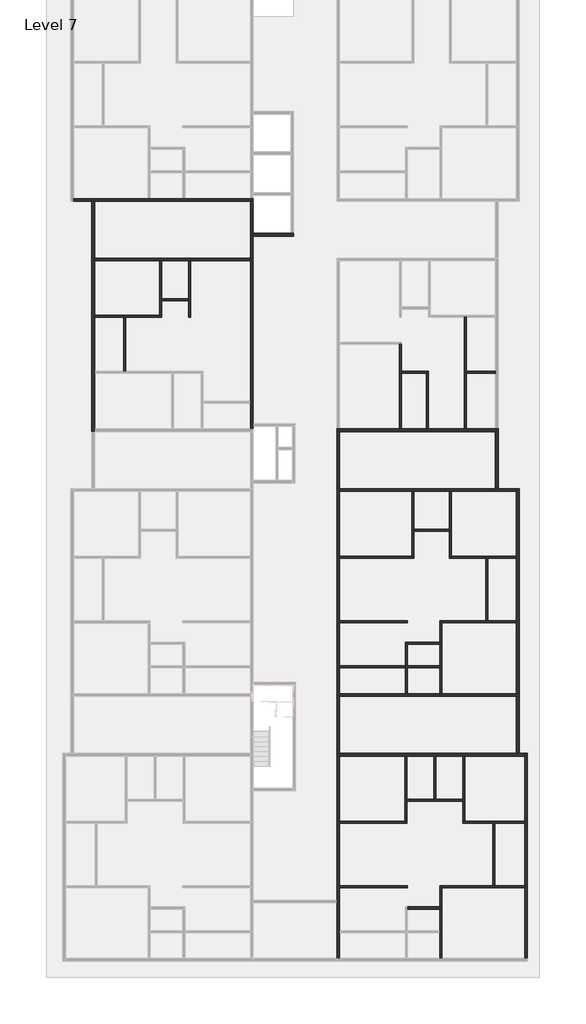
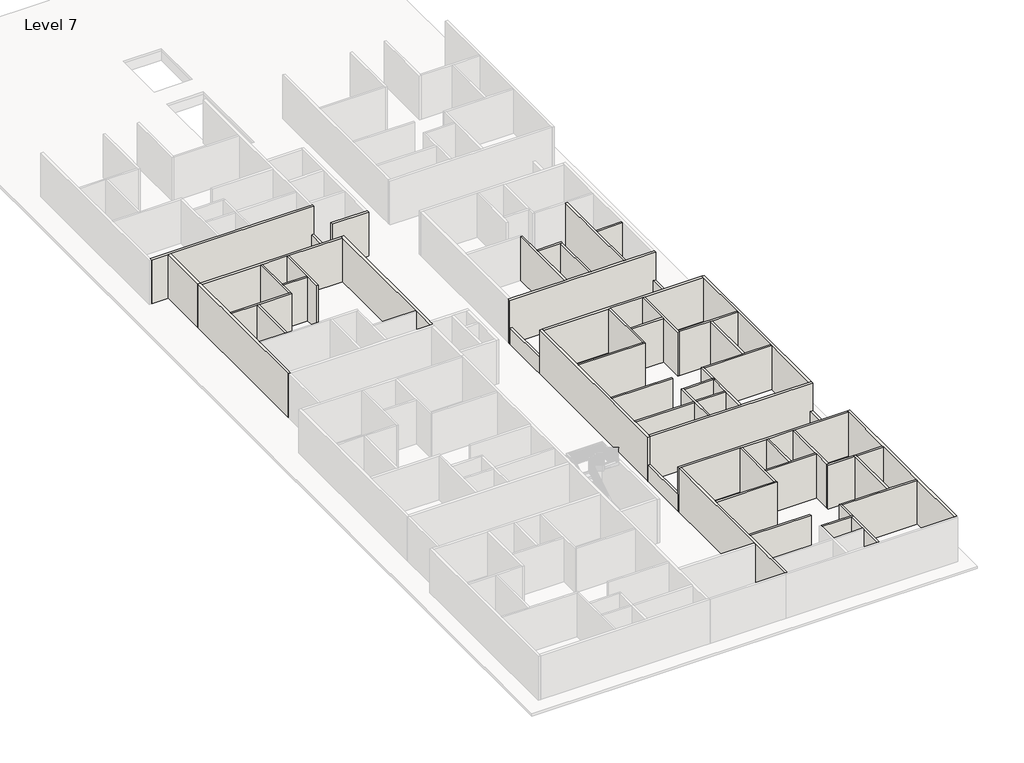
# One storey, part 2 of 8: 56 walls.
"""IFC4 building model written with IfcOpenShell, lengths in millimetres."""

from ifc_helpers import new_model, si_unit, frame, origin, place, context, project, spatial, polyline, outline, extrude, faceted_brep, element, save

model = new_model("IFC4")

# Units and contexts
model_context = context("Model", 3, world=origin())
ifc_project = project(units=[si_unit("LENGTHUNIT", "METRE", prefix="MILLI")], contexts=[model_context])

# Site, building, storey
site = spatial("IfcSite", under=ifc_project)
building = spatial("IfcBuilding", under=site)
storey = spatial("IfcBuildingStorey", under=building, Name="Level 7", Elevation=43522.6172466)

# Walls
placement = place(None, origin())
element("IfcWall", 1, ObjectType="4.5\"", at=placement, inside=storey, context=model_context, shape_type="Brep", body=[
    faceted_brep([(-12531.5544854, 2100.0216096, 43522.6172466), (-10907.2415084, 2100.0216096, 43522.6172466), (-10792.9415084, 2100.0216096, 43522.6172466), (-8759.6544854, 2100.0216096, 43522.6172466), (-8759.6544854, 2100.0216096, 46570.6172466), (-10792.9415084, 2100.0216096, 46570.6172466), (-10907.2415084, 2100.0216096, 46570.6172466), (-12531.5544854, 2100.0216096, 46570.6172466), (-12531.5544854, 2214.3216096, 43522.6172466), (-12531.5544854, 2214.3216096, 46570.6172466), (-8873.9544854, 2214.3216096, 46570.6172466), (-8759.6544854, 2214.3216096, 46570.6172466), (-8759.6544854, 2214.3216096, 43522.6172466), (-8873.9544854, 2214.3216096, 43522.6172466)], [[[0, 1, 2, 3, 4, 5, 6, 7]], [[8, 9, 10, 11, 12, 13]], [[3, 2, 1, 0, 8, 13, 12]], [[0, 7, 9, 8]], [[4, 3, 12, 11]], [[7, 6, 5, 4, 11, 10, 9]]]),
])
element("IfcWall", 2, ObjectType="4.5\"", at=placement, inside=storey, context=model_context, shape_type="Brep", body=[
    faceted_brep([(-8759.6544854, 2214.3216096, 43522.6172466), (-8759.6544854, 3014.4216096, 43522.6172466), (-8759.6544854, 3128.7216096, 43522.6172466), (-8759.6544854, 5264.2743917, 43522.6172466), (-8759.6544854, 5264.2743917, 46570.6172466), (-8759.6544854, 3128.7216096, 46570.6172466), (-8759.6544854, 3014.4216096, 46570.6172466), (-8759.6544854, 2214.3216096, 46570.6172466), (-8873.9544854, 2214.3216096, 43522.6172466), (-8873.9544854, 2214.3216096, 46570.6172466), (-8873.9544854, 5264.2743917, 46570.6172466), (-8873.9544854, 5264.2743917, 43522.6172466)], [[[0, 1, 2, 3, 4, 5, 6, 7]], [[8, 9, 10, 11]], [[3, 2, 1, 0, 8, 11]], [[0, 7, 9, 8]], [[4, 3, 11, 10]], [[7, 6, 5, 4, 10, 9]]]),
])
element("IfcWall", 3, ObjectType="4.5\"", at=placement, inside=storey, context=model_context, shape_type="Brep", body=[
    faceted_brep([(-7235.6544854, 5264.2743917, 43522.6172466), (-7235.6544854, 3128.7216096, 43522.6172466), (-7235.6544854, 3014.4216096, 43522.6172466), (-7235.6544854, 2100.0216096, 43522.6172466), (-7235.6544854, 2100.0216096, 46570.6172466), (-7235.6544854, 3014.4216096, 46570.6172466), (-7235.6544854, 3128.7216096, 46570.6172466), (-7235.6544854, 5264.2743917, 46570.6172466), (-7121.3544854, 5264.2743917, 43522.6172466), (-7121.3544854, 5264.2743917, 46570.6172466), (-7121.3544854, 2100.0216096, 46570.6172466), (-7121.3544854, 2100.0216096, 43522.6172466)], [[[0, 1, 2, 3, 4, 5, 6, 7]], [[8, 9, 10, 11]], [[3, 2, 1, 0, 8, 11]], [[4, 3, 11, 10]], [[0, 7, 9, 8]], [[7, 6, 5, 4, 10, 9]]]),
])
element("IfcWall", 4, ObjectType="4.5\"", at=placement, inside=storey, context=model_context, shape_type="SweptSolid", body=[
    extrude(outline(polyline([(-7235.6544854, 3014.4216096), (-8759.6544854, 3014.4216096), (-8759.6544854, 3128.7216096), (-7235.6544854, 3128.7216096), (-7235.6544854, 3014.4216096)])), frame((0.0, 0.0, 43522.6172466), z_axis=(0.0, 0.0, 1.0), x_axis=(1.0, 0.0, 0.0)), (0.0, 0.0, 1.0), 3048.0),
])
element("IfcWall", 5, ObjectType="4.5\"", at=placement, inside=storey, context=model_context, shape_type="SweptSolid", body=[
    extrude(outline(polyline([(-10907.2415084, -947.4344126), (-10907.2415084, 2100.0216096), (-10792.9415084, 2100.0216096), (-10792.9415084, -947.4344126), (-10907.2415084, -947.4344126)])), frame((0.0, 0.0, 43522.6172466), z_axis=(0.0, 0.0, 1.0), x_axis=(1.0, 0.0, 0.0)), (0.0, 0.0, 1.0), 3048.0),
])
element("IfcWall", 6, ObjectType="4.5\"", at=placement, inside=storey, context=model_context, shape_type="Brep", body=[
    faceted_brep([(5056.6584916, -31173.4344126, 43522.6172466), (6885.4584916, -31173.4344126, 43522.6172466), (6999.7584916, -31173.4344126, 43522.6172466), (6999.7584916, -31173.4344126, 46570.6172466), (6885.4584916, -31173.4344126, 46570.6172466), (5056.6584916, -31173.4344126, 46570.6172466), (5056.6584916, -31059.1344126, 43522.6172466), (5056.6584916, -31059.1344126, 46570.6172466), (6885.4584916, -31059.1344126, 46570.6172466), (6999.7584916, -31059.1344126, 46570.6172466), (6999.7584916, -31059.1344126, 43522.6172466), (6885.4584916, -31059.1344126, 43522.6172466)], [[[0, 1, 2, 3, 4, 5]], [[6, 7, 8, 9, 10, 11]], [[2, 1, 0, 6, 11, 10]], [[0, 5, 7, 6]], [[3, 2, 10, 9]], [[5, 4, 3, 9, 8, 7]]]),
])
element("IfcWall", 7, ObjectType="4.5\"", at=placement, inside=storey, context=model_context, shape_type="Brep", body=[
    faceted_brep([(6885.4584916, -31173.4344126, 43522.6172466), (6885.4584916, -32392.6344126, 43522.6172466), (6885.4584916, -32506.9344126, 43522.6172466), (6885.4584916, -33954.7344126, 43522.6172466), (6885.4584916, -33954.7344126, 46570.6172466), (6885.4584916, -32506.9344126, 46570.6172466), (6885.4584916, -32392.6344126, 46570.6172466), (6885.4584916, -31173.4344126, 46570.6172466), (6999.7584916, -31173.4344126, 43522.6172466), (6999.7584916, -31173.4344126, 46570.6172466), (6999.7584916, -33954.7344126, 46570.6172466), (6999.7584916, -33954.7344126, 43522.6172466)], [[[0, 1, 2, 3, 4, 5, 6, 7]], [[8, 9, 10, 11]], [[3, 2, 1, 0, 8, 11]], [[0, 7, 9, 8]], [[4, 3, 11, 10]], [[7, 6, 5, 4, 10, 9]]]),
])
element("IfcWall", 8, ObjectType="4.5\"", at=placement, inside=storey, context=model_context, shape_type="Brep", body=[
    faceted_brep([(6999.7584916, -31059.1344126, 43522.6172466), (6999.7584916, -29966.9344126, 43522.6172466), (6999.7584916, -29852.6344126, 43522.6172466), (6999.7584916, -29852.6344126, 46570.6172466), (6999.7584916, -29966.9344126, 46570.6172466), (6999.7584916, -31059.1344126, 46570.6172466), (6885.4584916, -31059.1344126, 43522.6172466), (6885.4584916, -31059.1344126, 46570.6172466), (6885.4584916, -29852.6344126, 46570.6172466), (6885.4584916, -29852.6344126, 43522.6172466)], [[[0, 1, 2, 3, 4, 5]], [[6, 7, 8, 9]], [[2, 1, 0, 6, 9]], [[0, 5, 7, 6]], [[3, 2, 9, 8]], [[5, 4, 3, 8, 7]]]),
])
element("IfcWall", 9, ObjectType="4.5\"", at=placement, inside=storey, context=model_context, shape_type="Brep", body=[
    faceted_brep([(6999.7584916, -29966.9344126, 43522.6172466), (11660.6584916, -29966.9344126, 43522.6172466), (11660.6584916, -29966.9344126, 46570.6172466), (6999.7584916, -29966.9344126, 46570.6172466), (6999.7584916, -29852.6344126, 43522.6172466), (6999.7584916, -29852.6344126, 46570.6172466), (9869.9584916, -29852.6344126, 46570.6172466), (9984.2584916, -29852.6344126, 46570.6172466), (11660.6584916, -29852.6344126, 46570.6172466), (11660.6584916, -29852.6344126, 43522.6172466), (9984.2584916, -29852.6344126, 43522.6172466), (9869.9584916, -29852.6344126, 43522.6172466)], [[[0, 1, 2, 3]], [[4, 5, 6, 7, 8, 9, 10, 11]], [[1, 0, 4, 11, 10, 9]], [[0, 3, 5, 4]], [[2, 1, 9, 8]], [[3, 2, 8, 7, 6, 5]]]),
])
element("IfcWall", 10, ObjectType="4.5\"", at=placement, inside=storey, context=model_context, shape_type="SweptSolid", body=[
    extrude(outline(polyline([(5056.6584916, -29966.9344126), (1259.3584916, -29966.9344126), (1259.3584916, -29852.6344126), (5056.6584916, -29852.6344126), (5056.6584916, -29966.9344126)])), frame((0.0, 0.0, 43522.6172466), z_axis=(0.0, 0.0, 1.0), x_axis=(1.0, 0.0, 0.0)), (0.0, 0.0, 1.0), 3048.0),
])
element("IfcWall", 11, ObjectType="4.5\"", at=placement, inside=storey, context=model_context, shape_type="Brep", body=[
    faceted_brep([(1259.3584916, -26347.4344126, 43522.6172466), (5031.2584916, -26347.4344126, 43522.6172466), (5031.2584916, -26347.4344126, 46570.6172466), (1259.3584916, -26347.4344126, 46570.6172466), (1259.3584916, -26233.1344126, 43522.6172466), (1259.3584916, -26233.1344126, 46570.6172466), (4916.9584916, -26233.1344126, 46570.6172466), (5031.2584916, -26233.1344126, 46570.6172466), (5031.2584916, -26233.1344126, 43522.6172466), (4916.9584916, -26233.1344126, 43522.6172466)], [[[0, 1, 2, 3]], [[4, 5, 6, 7, 8, 9]], [[1, 0, 4, 9, 8]], [[0, 3, 5, 4]], [[2, 1, 8, 7]], [[3, 2, 7, 6, 5]]]),
])
element("IfcWall", 12, ObjectType="4.5\"", at=placement, inside=storey, context=model_context, shape_type="Brep", body=[
    faceted_brep([(5031.2584916, -26233.1344126, 43522.6172466), (5031.2584916, -25128.2344126, 43522.6172466), (5031.2584916, -25013.9344126, 43522.6172466), (5031.2584916, -22575.5344126, 43522.6172466), (5031.2584916, -22575.5344126, 46570.6172466), (5031.2584916, -25013.9344126, 46570.6172466), (5031.2584916, -25128.2344126, 46570.6172466), (5031.2584916, -26233.1344126, 46570.6172466), (4916.9584916, -26233.1344126, 43522.6172466), (4916.9584916, -26233.1344126, 46570.6172466), (4916.9584916, -22575.5344126, 46570.6172466), (4916.9584916, -22575.5344126, 43522.6172466)], [[[0, 1, 2, 3, 4, 5, 6, 7]], [[8, 9, 10, 11]], [[3, 2, 1, 0, 8, 11]], [[0, 7, 9, 8]], [[4, 3, 11, 10]], [[7, 6, 5, 4, 10, 9]]]),
])
element("IfcWall", 13, ObjectType="4.5\"", at=placement, inside=storey, context=model_context, shape_type="Brep", body=[
    faceted_brep([(9984.2584916, -29852.6344126, 43522.6172466), (9984.2584916, -26347.4344126, 43522.6172466), (9984.2584916, -26233.1344126, 43522.6172466), (9984.2584916, -26233.1344126, 46570.6172466), (9984.2584916, -26347.4344126, 46570.6172466), (9984.2584916, -29852.6344126, 46570.6172466), (9869.9584916, -29852.6344126, 43522.6172466), (9869.9584916, -29852.6344126, 46570.6172466), (9869.9584916, -26347.4344126, 46570.6172466), (9869.9584916, -26233.1344126, 46570.6172466), (9869.9584916, -26233.1344126, 43522.6172466), (9869.9584916, -26347.4344126, 43522.6172466)], [[[0, 1, 2, 3, 4, 5]], [[6, 7, 8, 9, 10, 11]], [[2, 1, 0, 6, 11, 10]], [[0, 5, 7, 6]], [[3, 2, 10, 9]], [[5, 4, 3, 9, 8, 7]]]),
])
element("IfcWall", 14, ObjectType="4.5\"", at=placement, inside=storey, context=model_context, shape_type="SweptSolid", body=[
    extrude(outline(polyline([(11660.6584916, -26347.4344126), (9984.2584916, -26347.4344126), (9984.2584916, -26233.1344126), (11660.6584916, -26233.1344126), (11660.6584916, -26347.4344126)])), frame((0.0, 0.0, 43522.6172466), z_axis=(0.0, 0.0, 1.0), x_axis=(1.0, 0.0, 0.0)), (0.0, 0.0, 1.0), 3048.0),
])
element("IfcWall", 15, ObjectType="4.5\"", at=placement, inside=storey, context=model_context, shape_type="Brep", body=[
    faceted_brep([(9869.9584916, -26233.1344126, 43522.6172466), (8307.8584916, -26233.1344126, 43522.6172466), (8193.5584916, -26233.1344126, 43522.6172466), (8193.5584916, -26233.1344126, 46570.6172466), (8307.8584916, -26233.1344126, 46570.6172466), (9869.9584916, -26233.1344126, 46570.6172466), (9869.9584916, -26347.4344126, 43522.6172466), (9869.9584916, -26347.4344126, 46570.6172466), (8193.5584916, -26347.4344126, 46570.6172466), (8193.5584916, -26347.4344126, 43522.6172466)], [[[0, 1, 2, 3, 4, 5]], [[6, 7, 8, 9]], [[2, 1, 0, 6, 9]], [[0, 5, 7, 6]], [[3, 2, 9, 8]], [[5, 4, 3, 8, 7]]]),
])
element("IfcWall", 16, ObjectType="4.5\"", at=placement, inside=storey, context=model_context, shape_type="Brep", body=[
    faceted_brep([(8307.8584916, -26233.1344126, 43522.6172466), (8307.8584916, -22575.5344126, 43522.6172466), (8307.8584916, -22575.5344126, 46570.6172466), (8307.8584916, -26233.1344126, 46570.6172466), (8193.5584916, -26233.1344126, 43522.6172466), (8193.5584916, -26233.1344126, 46570.6172466), (8193.5584916, -25128.2344126, 46570.6172466), (8193.5584916, -25013.9344126, 46570.6172466), (8193.5584916, -22575.5344126, 46570.6172466), (8193.5584916, -22575.5344126, 43522.6172466), (8193.5584916, -25013.9344126, 43522.6172466), (8193.5584916, -25128.2344126, 43522.6172466)], [[[0, 1, 2, 3]], [[4, 5, 6, 7, 8, 9, 10, 11]], [[1, 0, 4, 11, 10, 9]], [[0, 3, 5, 4]], [[2, 1, 9, 8]], [[3, 2, 8, 7, 6, 5]]]),
])
element("IfcWall", 17, ObjectType="4.5\"", at=placement, inside=storey, context=model_context, shape_type="Brep", body=[
    faceted_brep([(5031.2584916, -25128.2344126, 43522.6172466), (8193.5584916, -25128.2344126, 43522.6172466), (8193.5584916, -25128.2344126, 46570.6172466), (5031.2584916, -25128.2344126, 46570.6172466), (5031.2584916, -25013.9344126, 43522.6172466), (5031.2584916, -25013.9344126, 46570.6172466), (6555.2584916, -25013.9344126, 46570.6172466), (6669.5584916, -25013.9344126, 46570.6172466), (8193.5584916, -25013.9344126, 46570.6172466), (8193.5584916, -25013.9344126, 43522.6172466), (6669.5584916, -25013.9344126, 43522.6172466), (6555.2584916, -25013.9344126, 43522.6172466)], [[[0, 1, 2, 3]], [[4, 5, 6, 7, 8, 9, 10, 11]], [[1, 0, 4, 11, 10, 9]], [[0, 3, 5, 4]], [[2, 1, 9, 8]], [[3, 2, 8, 7, 6, 5]]]),
])
element("IfcWall", 18, ObjectType="4.5\"", at=placement, inside=storey, context=model_context, shape_type="SweptSolid", body=[
    extrude(outline(polyline([(6555.2584916, -25013.9344126), (6555.2584916, -22575.5344126), (6669.5584916, -22575.5344126), (6669.5584916, -25013.9344126), (6555.2584916, -25013.9344126)])), frame((0.0, 0.0, 43522.6172466), z_axis=(0.0, 0.0, 1.0), x_axis=(1.0, 0.0, 0.0)), (0.0, 0.0, 1.0), 3048.0),
])
element("IfcWall", 19, ObjectType="4.5\"", at=placement, inside=storey, context=model_context, shape_type="SweptSolid", body=[
    extrude(outline(polyline([(4942.3584916, -17622.5344126), (1259.3584916, -17622.5344126), (1259.3584916, -17508.2344126), (4942.3584916, -17508.2344126), (4942.3584916, -17622.5344126)])), frame((0.0, 0.0, 43522.6172466), z_axis=(0.0, 0.0, 1.0), x_axis=(1.0, 0.0, 0.0)), (0.0, 0.0, 1.0), 3048.0),
])
element("IfcWall", 20, ObjectType="4.5\"", at=placement, inside=storey, context=model_context, shape_type="Brep", body=[
    faceted_brep([(4942.3584916, -16174.7344126, 43522.6172466), (4942.3584916, -17508.2344126, 43522.6172466), (4942.3584916, -17622.5344126, 43522.6172466), (4942.3584916, -19070.3344126, 43522.6172466), (4942.3584916, -19070.3344126, 46570.6172466), (4942.3584916, -17622.5344126, 46570.6172466), (4942.3584916, -17508.2344126, 46570.6172466), (4942.3584916, -16174.7344126, 46570.6172466), (5056.6584916, -16174.7344126, 43522.6172466), (5056.6584916, -16174.7344126, 46570.6172466), (5056.6584916, -16289.0344126, 46570.6172466), (5056.6584916, -17508.2344126, 46570.6172466), (5056.6584916, -17622.5344126, 46570.6172466), (5056.6584916, -19070.3344126, 46570.6172466), (5056.6584916, -19070.3344126, 43522.6172466), (5056.6584916, -17622.5344126, 43522.6172466), (5056.6584916, -17508.2344126, 43522.6172466), (5056.6584916, -16289.0344126, 43522.6172466)], [[[0, 1, 2, 3, 4, 5, 6, 7]], [[8, 9, 10, 11, 12, 13, 14, 15, 16, 17]], [[3, 2, 1, 0, 8, 17, 16, 15, 14]], [[4, 3, 14, 13]], [[0, 7, 9, 8]], [[7, 6, 5, 4, 13, 12, 11, 10, 9]]]),
])
element("IfcWall", 21, ObjectType="4.5\"", at=placement, inside=storey, context=model_context, shape_type="Brep", body=[
    faceted_brep([(5056.6584916, -16289.0344126, 43522.6172466), (6885.4584916, -16289.0344126, 43522.6172466), (6999.7584916, -16289.0344126, 43522.6172466), (6999.7584916, -16289.0344126, 46570.6172466), (6885.4584916, -16289.0344126, 46570.6172466), (5056.6584916, -16289.0344126, 46570.6172466), (5056.6584916, -16174.7344126, 43522.6172466), (5056.6584916, -16174.7344126, 46570.6172466), (6885.4584916, -16174.7344126, 46570.6172466), (6999.7584916, -16174.7344126, 46570.6172466), (6999.7584916, -16174.7344126, 43522.6172466), (6885.4584916, -16174.7344126, 43522.6172466)], [[[0, 1, 2, 3, 4, 5]], [[6, 7, 8, 9, 10, 11]], [[2, 1, 0, 6, 11, 10]], [[0, 5, 7, 6]], [[3, 2, 10, 9]], [[5, 4, 3, 9, 8, 7]]]),
])
element("IfcWall", 22, ObjectType="4.5\"", at=placement, inside=storey, context=model_context, shape_type="Brep", body=[
    faceted_brep([(6885.4584916, -16289.0344126, 43522.6172466), (6885.4584916, -17508.2344126, 43522.6172466), (6885.4584916, -17622.5344126, 43522.6172466), (6885.4584916, -19070.3344126, 43522.6172466), (6885.4584916, -19070.3344126, 46570.6172466), (6885.4584916, -17622.5344126, 46570.6172466), (6885.4584916, -17508.2344126, 46570.6172466), (6885.4584916, -16289.0344126, 46570.6172466), (6999.7584916, -16289.0344126, 43522.6172466), (6999.7584916, -16289.0344126, 46570.6172466), (6999.7584916, -19070.3344126, 46570.6172466), (6999.7584916, -19070.3344126, 43522.6172466)], [[[0, 1, 2, 3, 4, 5, 6, 7]], [[8, 9, 10, 11]], [[3, 2, 1, 0, 8, 11]], [[0, 7, 9, 8]], [[4, 3, 11, 10]], [[7, 6, 5, 4, 10, 9]]]),
])
element("IfcWall", 23, ObjectType="4.5\"", at=placement, inside=storey, context=model_context, shape_type="SweptSolid", body=[
    extrude(outline(polyline([(6885.4584916, -17622.5344126), (5056.6584916, -17622.5344126), (5056.6584916, -17508.2344126), (6885.4584916, -17508.2344126), (6885.4584916, -17622.5344126)])), frame((0.0, 0.0, 43522.6172466), z_axis=(0.0, 0.0, 1.0), x_axis=(1.0, 0.0, 0.0)), (0.0, 0.0, 1.0), 3048.0),
])
element("IfcWall", 24, ObjectType="4.5\"", at=placement, inside=storey, context=model_context, shape_type="Brep", body=[
    faceted_brep([(6999.7584916, -16174.7344126, 43522.6172466), (6999.7584916, -15082.5344126, 43522.6172466), (6999.7584916, -14968.2344126, 43522.6172466), (6999.7584916, -14968.2344126, 46570.6172466), (6999.7584916, -15082.5344126, 46570.6172466), (6999.7584916, -16174.7344126, 46570.6172466), (6885.4584916, -16174.7344126, 43522.6172466), (6885.4584916, -16174.7344126, 46570.6172466), (6885.4584916, -14968.2344126, 46570.6172466), (6885.4584916, -14968.2344126, 43522.6172466)], [[[0, 1, 2, 3, 4, 5]], [[6, 7, 8, 9]], [[2, 1, 0, 6, 9]], [[0, 5, 7, 6]], [[3, 2, 9, 8]], [[5, 4, 3, 8, 7]]]),
])
element("IfcWall", 25, ObjectType="4.5\"", at=placement, inside=storey, context=model_context, shape_type="Brep", body=[
    faceted_brep([(6999.7584916, -15082.5344126, 43522.6172466), (11208.5214687, -15082.5344126, 43522.6172466), (11208.5214687, -15082.5344126, 46570.6172466), (6999.7584916, -15082.5344126, 46570.6172466), (6999.7584916, -14968.2344126, 43522.6172466), (6999.7584916, -14968.2344126, 46570.6172466), (9469.9084916, -14968.2344126, 46570.6172466), (9584.2084916, -14968.2344126, 46570.6172466), (11208.5214687, -14968.2344126, 46570.6172466), (11208.5214687, -14968.2344126, 43522.6172466), (9584.2084916, -14968.2344126, 43522.6172466), (9469.9084916, -14968.2344126, 43522.6172466)], [[[0, 1, 2, 3]], [[4, 5, 6, 7, 8, 9, 10, 11]], [[1, 0, 4, 11, 10, 9]], [[0, 3, 5, 4]], [[2, 1, 9, 8]], [[3, 2, 8, 7, 6, 5]]]),
])
element("IfcWall", 26, ObjectType="4.5\"", at=placement, inside=storey, context=model_context, shape_type="SweptSolid", body=[
    extrude(outline(polyline([(5056.6584916, -15082.5344126), (1259.3584916, -15082.5344126), (1259.3584916, -14968.2344126), (5056.6584916, -14968.2344126), (5056.6584916, -15082.5344126)])), frame((0.0, 0.0, 43522.6172466), z_axis=(0.0, 0.0, 1.0), x_axis=(1.0, 0.0, 0.0)), (0.0, 0.0, 1.0), 3048.0),
])
element("IfcWall", 27, ObjectType="4.5\"", at=placement, inside=storey, context=model_context, shape_type="Brep", body=[
    faceted_brep([(1259.3584916, -11463.0344126, 43522.6172466), (5430.0214687, -11463.0344126, 43522.6172466), (5430.0214687, -11463.0344126, 46570.6172466), (1259.3584916, -11463.0344126, 46570.6172466), (1259.3584916, -11348.7344126, 43522.6172466), (1259.3584916, -11348.7344126, 46570.6172466), (5315.7214687, -11348.7344126, 46570.6172466), (5430.0214687, -11348.7344126, 46570.6172466), (5430.0214687, -11348.7344126, 43522.6172466), (5315.7214687, -11348.7344126, 43522.6172466)], [[[0, 1, 2, 3]], [[4, 5, 6, 7, 8, 9]], [[1, 0, 4, 9, 8]], [[0, 3, 5, 4]], [[2, 1, 8, 7]], [[3, 2, 7, 6, 5]]]),
])
element("IfcWall", 28, ObjectType="4.5\"", at=placement, inside=storey, context=model_context, shape_type="Brep", body=[
    faceted_brep([(5430.0214687, -11348.7344126, 43522.6172466), (5430.0214687, -9939.0344126, 43522.6172466), (5430.0214687, -9824.7344126, 43522.6172466), (5430.0214687, -7691.1344126, 43522.6172466), (5430.0214687, -7691.1344126, 46570.6172466), (5430.0214687, -9824.7344126, 46570.6172466), (5430.0214687, -9939.0344126, 46570.6172466), (5430.0214687, -11348.7344126, 46570.6172466), (5315.7214687, -11348.7344126, 43522.6172466), (5315.7214687, -11348.7344126, 46570.6172466), (5315.7214687, -7691.1344126, 46570.6172466), (5315.7214687, -7691.1344126, 43522.6172466)], [[[0, 1, 2, 3, 4, 5, 6, 7]], [[8, 9, 10, 11]], [[3, 2, 1, 0, 8, 11]], [[0, 7, 9, 8]], [[4, 3, 11, 10]], [[7, 6, 5, 4, 10, 9]]]),
])
element("IfcWall", 29, ObjectType="4.5\"", at=placement, inside=storey, context=model_context, shape_type="SweptSolid", body=[
    extrude(outline(polyline([(7436.6214687, -9939.0344126), (5430.0214687, -9939.0344126), (5430.0214687, -9824.7344126), (7436.6214687, -9824.7344126), (7436.6214687, -9939.0344126)])), frame((0.0, 0.0, 43522.6172466), z_axis=(0.0, 0.0, 1.0), x_axis=(1.0, 0.0, 0.0)), (0.0, 0.0, 1.0), 3048.0),
])
element("IfcWall", 30, ObjectType="4.5\"", at=placement, inside=storey, context=model_context, shape_type="Brep", body=[
    faceted_brep([(7436.6214687, -7691.1344126, 43522.6172466), (7436.6214687, -9824.7344126, 43522.6172466), (7436.6214687, -9939.0344126, 43522.6172466), (7436.6214687, -11463.0344126, 43522.6172466), (7436.6214687, -11463.0344126, 46570.6172466), (7436.6214687, -9939.0344126, 46570.6172466), (7436.6214687, -9824.7344126, 46570.6172466), (7436.6214687, -7691.1344126, 46570.6172466), (7550.9214687, -7691.1344126, 43522.6172466), (7550.9214687, -7691.1344126, 46570.6172466), (7550.9214687, -11348.7344126, 46570.6172466), (7550.9214687, -11463.0344126, 46570.6172466), (7550.9214687, -11463.0344126, 43522.6172466), (7550.9214687, -11348.7344126, 43522.6172466)], [[[0, 1, 2, 3, 4, 5, 6, 7]], [[8, 9, 10, 11, 12, 13]], [[3, 2, 1, 0, 8, 13, 12]], [[0, 7, 9, 8]], [[4, 3, 12, 11]], [[7, 6, 5, 4, 11, 10, 9]]]),
])
element("IfcWall", 31, ObjectType="4.5\"", at=placement, inside=storey, context=model_context, shape_type="Brep", body=[
    faceted_brep([(7550.9214687, -11463.0344126, 43522.6172466), (9469.9084916, -11463.0344126, 43522.6172466), (9584.2084916, -11463.0344126, 43522.6172466), (11208.5214687, -11463.0344126, 43522.6172466), (11208.5214687, -11463.0344126, 46570.6172466), (9584.2084916, -11463.0344126, 46570.6172466), (9469.9084916, -11463.0344126, 46570.6172466), (7550.9214687, -11463.0344126, 46570.6172466), (7550.9214687, -11348.7344126, 43522.6172466), (7550.9214687, -11348.7344126, 46570.6172466), (11208.5214687, -11348.7344126, 46570.6172466), (11208.5214687, -11348.7344126, 43522.6172466)], [[[0, 1, 2, 3, 4, 5, 6, 7]], [[8, 9, 10, 11]], [[3, 2, 1, 0, 8, 11]], [[0, 7, 9, 8]], [[4, 3, 11, 10]], [[7, 6, 5, 4, 10, 9]]]),
])
element("IfcWall", 32, ObjectType="4.5\"", at=placement, inside=storey, context=model_context, shape_type="SweptSolid", body=[
    extrude(outline(polyline([(9469.9084916, -14968.2344126), (9469.9084916, -11463.0344126), (9584.2084916, -11463.0344126), (9584.2084916, -14968.2344126), (9469.9084916, -14968.2344126)])), frame((0.0, 0.0, 43522.6172466), z_axis=(0.0, 0.0, 1.0), x_axis=(1.0, 0.0, 0.0)), (0.0, 0.0, 1.0), 3048.0),
])
element("IfcWall", 33, ObjectType="4.5\"", at=placement, inside=storey, context=model_context, shape_type="Brep", body=[
    faceted_brep([(4610.8714687, 572.7745083, 43522.6172466), (4610.8714687, -4185.9344126, 43522.6172466), (4610.8714687, -4185.9344126, 46570.6172466), (4610.8714687, 572.7745083, 46570.6172466), (4725.1714687, 572.7745083, 43522.6172466), (4725.1714687, 572.7745083, 46570.6172466), (4725.1714687, -947.4344126, 46570.6172466), (4725.1714687, -1061.7344126, 46570.6172466), (4725.1714687, -4185.9344126, 46570.6172466), (4725.1714687, -4185.9344126, 43522.6172466), (4725.1714687, -1061.7344126, 43522.6172466), (4725.1714687, -947.4344126, 43522.6172466)], [[[0, 1, 2, 3]], [[4, 5, 6, 7, 8, 9, 10, 11]], [[1, 0, 4, 11, 10, 9]], [[0, 3, 5, 4]], [[2, 1, 9, 8]], [[3, 2, 8, 7, 6, 5]]]),
])
element("IfcWall", 34, ObjectType="4.5\"", at=placement, inside=storey, context=model_context, shape_type="Brep", body=[
    faceted_brep([(4725.1714687, -1061.7344126, 43522.6172466), (6134.8714687, -1061.7344126, 43522.6172466), (6249.1714687, -1061.7344126, 43522.6172466), (6249.1714687, -1061.7344126, 46570.6172466), (6134.8714687, -1061.7344126, 46570.6172466), (4725.1714687, -1061.7344126, 46570.6172466), (4725.1714687, -947.4344126, 43522.6172466), (4725.1714687, -947.4344126, 46570.6172466), (6249.1714687, -947.4344126, 46570.6172466), (6249.1714687, -947.4344126, 43522.6172466)], [[[0, 1, 2, 3, 4, 5]], [[6, 7, 8, 9]], [[2, 1, 0, 6, 9]], [[0, 5, 7, 6]], [[3, 2, 9, 8]], [[5, 4, 3, 8, 7]]]),
])
element("IfcWall", 35, ObjectType="4.5\"", at=placement, inside=storey, context=model_context, shape_type="SweptSolid", body=[
    extrude(outline(polyline([(6134.8714687, -4185.9344126), (6134.8714687, -1061.7344126), (6249.1714687, -1061.7344126), (6249.1714687, -4185.9344126), (6134.8714687, -4185.9344126)])), frame((0.0, 0.0, 43522.6172466), z_axis=(0.0, 0.0, 1.0), x_axis=(1.0, 0.0, 0.0)), (0.0, 0.0, 1.0), 3048.0),
])
element("IfcWall", 36, ObjectType="4.5\"", at=placement, inside=storey, context=model_context, shape_type="Brep", body=[
    faceted_brep([(8396.7584916, -4185.9344126, 43522.6172466), (8396.7584916, -1061.7344126, 43522.6172466), (8396.7584916, -947.4344126, 43522.6172466), (8396.7584916, 2100.0216096, 43522.6172466), (8396.7584916, 2100.0216096, 46570.6172466), (8396.7584916, -947.4344126, 46570.6172466), (8396.7584916, -1061.7344126, 46570.6172466), (8396.7584916, -4185.9344126, 46570.6172466), (8282.4584916, -4185.9344126, 43522.6172466), (8282.4584916, -4185.9344126, 46570.6172466), (8282.4584916, 2100.0216096, 46570.6172466), (8282.4584916, 2100.0216096, 43522.6172466)], [[[0, 1, 2, 3, 4, 5, 6, 7]], [[8, 9, 10, 11]], [[3, 2, 1, 0, 8, 11]], [[0, 7, 9, 8]], [[4, 3, 11, 10]], [[7, 6, 5, 4, 10, 9]]]),
])
element("IfcWall", 37, ObjectType="4.5\"", at=placement, inside=storey, context=model_context, shape_type="SweptSolid", body=[
    extrude(outline(polyline([(8396.7584916, -947.4344126), (10021.0714687, -947.4344126), (10021.0714687, -1061.7344126), (8396.7584916, -1061.7344126), (8396.7584916, -947.4344126)])), frame((0.0, 0.0, 43522.6172466), z_axis=(0.0, 0.0, 1.0), x_axis=(1.0, 0.0, 0.0)), (0.0, 0.0, 1.0), 3048.0),
])
element("IfcWall", 38, ObjectType="6\"", at=placement, inside=storey, context=model_context, shape_type="Brep", body=[
    faceted_brep([(-13719.0044854, 8615.1216096, 43522.6172466), (-12683.9544854, 8615.1216096, 43522.6172466), (-12531.5544854, 8615.1216096, 43522.6172466), (-3769.8415084, 8615.1216096, 43522.6172466), (-3617.4415084, 8615.1216096, 43522.6172466), (-3617.4415084, 8615.1216096, 44741.8172466), (-3617.4415084, 8615.1216096, 46570.6172466), (-12531.5544854, 8615.1216096, 46570.6172466), (-12683.9544854, 8615.1216096, 46570.6172466), (-13719.0044854, 8615.1216096, 46570.6172466), (-13719.0044854, 8767.5216096, 43522.6172466), (-13719.0044854, 8767.5216096, 46570.6172466), (-9510.2415084, 8767.5216096, 46570.6172466), (-9395.9415084, 8767.5216096, 46570.6172466), (-7567.1415084, 8767.5216096, 46570.6172466), (-7452.8415084, 8767.5216096, 46570.6172466), (-3769.8415084, 8767.5216096, 46570.6172466), (-3617.4415084, 8767.5216096, 46570.6172466), (-3617.4415084, 8767.5216096, 43522.6172466), (-3769.8415084, 8767.5216096, 43522.6172466), (-7452.8415084, 8767.5216096, 43522.6172466), (-7567.1415084, 8767.5216096, 43522.6172466), (-9395.9415084, 8767.5216096, 43522.6172466), (-9510.2415084, 8767.5216096, 43522.6172466)], [[[0, 1, 2, 3, 4, 5, 6, 7, 8, 9]], [[10, 11, 12, 13, 14, 15, 16, 17, 18, 19, 20, 21, 22, 23]], [[4, 3, 2, 1, 0, 10, 23, 22, 21, 20, 19, 18]], [[0, 9, 11, 10]], [[4, 18, 17, 6, 5]], [[9, 8, 7, 6, 17, 16, 15, 14, 13, 12, 11]]]),
])
element("IfcWall", 39, ObjectType="6\"", at=placement, inside=storey, context=model_context, shape_type="Brep", body=[
    faceted_brep([(-12683.9544854, 5416.6743917, 43522.6172466), (-12683.9544854, -4338.3344126, 43522.6172466), (-12683.9544854, -4338.3344126, 46570.6172466), (-12683.9544854, 5416.6743917, 46570.6172466), (-12531.5544854, 5416.6743917, 43522.6172466), (-12531.5544854, 5416.6743917, 46570.6172466), (-12531.5544854, 5264.2743917, 46570.6172466), (-12531.5544854, 2214.3216096, 46570.6172466), (-12531.5544854, 2100.0216096, 46570.6172466), (-12531.5544854, -947.4344126, 46570.6172466), (-12531.5544854, -1061.7344126, 46570.6172466), (-12531.5544854, -4185.9344126, 46570.6172466), (-12531.5544854, -4338.3344126, 46570.6172466), (-12531.5544854, -4338.3344126, 43522.6172466), (-12531.5544854, -4185.9344126, 43522.6172466), (-12531.5544854, -1061.7344126, 43522.6172466), (-12531.5544854, -947.4344126, 43522.6172466), (-12531.5544854, 2100.0216096, 43522.6172466), (-12531.5544854, 2214.3216096, 43522.6172466), (-12531.5544854, 5264.2743917, 43522.6172466)], [[[0, 1, 2, 3]], [[4, 5, 6, 7, 8, 9, 10, 11, 12, 13, 14, 15, 16, 17, 18, 19]], [[1, 0, 4, 19, 18, 17, 16, 15, 14, 13]], [[2, 1, 13, 12]], [[0, 3, 5, 4]], [[3, 2, 12, 11, 10, 9, 8, 7, 6, 5]]]),
])
element("IfcWall", 40, ObjectType="6\"", at=placement, inside=storey, context=model_context, shape_type="Brep", body=[
    faceted_brep([(-3617.4415084, -4185.9344126, 43522.6172466), (-3617.4415084, -4034.6751812, 43522.6172466), (-3617.4415084, -3882.2751812, 43522.6172466), (-3617.4415084, 5416.6743917, 43522.6172466), (-3617.4415084, 5416.6743917, 46570.6172466), (-3617.4415084, -3882.2751812, 46570.6172466), (-3617.4415084, -4034.6751812, 46570.6172466), (-3617.4415084, -4185.9344126, 46570.6172466), (-3769.8415084, -4185.9344126, 43522.6172466), (-3769.8415084, -4185.9344126, 46570.6172466), (-3769.8415084, -2738.1344126, 46570.6172466), (-3769.8415084, -2623.8344126, 46570.6172466), (-3769.8415084, 5264.2743917, 46570.6172466), (-3769.8415084, 5416.6743917, 46570.6172466), (-3769.8415084, 5416.6743917, 43522.6172466), (-3769.8415084, 5264.2743917, 43522.6172466), (-3769.8415084, -2623.8344126, 43522.6172466), (-3769.8415084, -2738.1344126, 43522.6172466)], [[[0, 1, 2, 3, 4, 5, 6, 7]], [[8, 9, 10, 11, 12, 13, 14, 15, 16, 17]], [[3, 2, 1, 0, 8, 17, 16, 15, 14]], [[0, 7, 9, 8]], [[3, 14, 13, 4]], [[7, 6, 5, 4, 13, 12, 11, 10, 9]]]),
])
element("IfcWall", 41, ObjectType="6\"", at=placement, inside=storey, context=model_context, shape_type="Brep", body=[
    faceted_brep([(-3769.8415084, 5416.6743917, 46570.6172466), (-3769.8415084, 5416.6743917, 43522.6172466), (-12531.5544854, 5416.6743917, 43522.6172466), (-12531.5544854, 5416.6743917, 46570.6172466), (-3769.8415084, 5264.2743917, 43522.6172466), (-3769.8415084, 5264.2743917, 46570.6172466), (-7121.3544854, 5264.2743917, 46570.6172466), (-7235.6544854, 5264.2743917, 46570.6172466), (-8759.6544854, 5264.2743917, 46570.6172466), (-8873.9544854, 5264.2743917, 46570.6172466), (-12531.5544854, 5264.2743917, 46570.6172466), (-12531.5544854, 5264.2743917, 43522.6172466), (-8873.9544854, 5264.2743917, 43522.6172466), (-8759.6544854, 5264.2743917, 43522.6172466), (-7235.6544854, 5264.2743917, 43522.6172466), (-7121.3544854, 5264.2743917, 43522.6172466)], [[[0, 1, 2, 3]], [[4, 5, 6, 7, 8, 9, 10, 11, 12, 13, 14, 15]], [[2, 1, 4, 15, 14, 13, 12, 11]], [[3, 2, 11, 10]], [[0, 5, 4, 1]], [[0, 3, 10, 9, 8, 7, 6, 5]]]),
])
element("IfcWall", 42, ObjectType="6\"", at=placement, inside=storey, context=model_context, shape_type="Brep", body=[
    faceted_brep([(11813.0584916, -33954.7344126, 43522.6172466), (11813.0584916, -22423.1344126, 43522.6172466), (11813.0584916, -22423.1344126, 46570.6172466), (11813.0584916, -33954.7344126, 46570.6172466), (11660.6584916, -33954.7344126, 43522.6172466), (11660.6584916, -33954.7344126, 46570.6172466), (11660.6584916, -29966.9344126, 46570.6172466), (11660.6584916, -29852.6344126, 46570.6172466), (11660.6584916, -26347.4344126, 46570.6172466), (11660.6584916, -26233.1344126, 46570.6172466), (11660.6584916, -22575.5344126, 46570.6172466), (11660.6584916, -22423.1344126, 46570.6172466), (11660.6584916, -22423.1344126, 43522.6172466), (11660.6584916, -22575.5344126, 43522.6172466), (11660.6584916, -26233.1344126, 43522.6172466), (11660.6584916, -26347.4344126, 43522.6172466), (11660.6584916, -29852.6344126, 43522.6172466), (11660.6584916, -29966.9344126, 43522.6172466)], [[[0, 1, 2, 3]], [[4, 5, 6, 7, 8, 9, 10, 11, 12, 13, 14, 15, 16, 17]], [[1, 0, 4, 17, 16, 15, 14, 13, 12]], [[0, 3, 5, 4]], [[2, 1, 12, 11]], [[3, 2, 11, 10, 9, 8, 7, 6, 5]]]),
])
element("IfcWall", 43, ObjectType="6\"", at=placement, inside=storey, context=model_context, shape_type="Brep", body=[
    faceted_brep([(11660.6584916, -22423.1344126, 43522.6172466), (11360.9214687, -22423.1344126, 43522.6172466), (11208.5214687, -22423.1344126, 43522.6172466), (1259.3584916, -22423.1344126, 43522.6172466), (1106.9584916, -22423.1344126, 43522.6172466), (1106.9584916, -22423.1344126, 44741.8172466), (1106.9584916, -22423.1344126, 46570.6172466), (11660.6584916, -22423.1344126, 46570.6172466), (11660.6584916, -22575.5344126, 43522.6172466), (11660.6584916, -22575.5344126, 46570.6172466), (8307.8584916, -22575.5344126, 46570.6172466), (8193.5584916, -22575.5344126, 46570.6172466), (6669.5584916, -22575.5344126, 46570.6172466), (6555.2584916, -22575.5344126, 46570.6172466), (5031.2584916, -22575.5344126, 46570.6172466), (4916.9584916, -22575.5344126, 46570.6172466), (1259.3584916, -22575.5344126, 46570.6172466), (1106.9584916, -22575.5344126, 46570.6172466), (1106.9584916, -22575.5344126, 43522.6172466), (1259.3584916, -22575.5344126, 43522.6172466), (4916.9584916, -22575.5344126, 43522.6172466), (5031.2584916, -22575.5344126, 43522.6172466), (6555.2584916, -22575.5344126, 43522.6172466), (6669.5584916, -22575.5344126, 43522.6172466), (8193.5584916, -22575.5344126, 43522.6172466), (8307.8584916, -22575.5344126, 43522.6172466)], [[[0, 1, 2, 3, 4, 5, 6, 7]], [[8, 9, 10, 11, 12, 13, 14, 15, 16, 17, 18, 19, 20, 21, 22, 23, 24, 25]], [[4, 3, 2, 1, 0, 8, 25, 24, 23, 22, 21, 20, 19, 18]], [[0, 7, 9, 8]], [[4, 18, 17, 6, 5]], [[7, 6, 17, 16, 15, 14, 13, 12, 11, 10, 9]]]),
])
element("IfcWall", 44, ObjectType="6\"", at=placement, inside=storey, context=model_context, shape_type="Brep", body=[
    faceted_brep([(1106.9584916, -22575.5344126, 46570.6172466), (1106.9584916, -22575.5344126, 43522.6172466), (1106.9584916, -30668.5325185, 43522.6172466), (1106.9584916, -30820.9325185, 43522.6172466), (1106.9584916, -33954.7344126, 43522.6172466), (1106.9584916, -33954.7344126, 46570.6172466), (1106.9584916, -30820.9325185, 46570.6172466), (1106.9584916, -30668.5325185, 46570.6172466), (1259.3584916, -22575.5344126, 43522.6172466), (1259.3584916, -22575.5344126, 46570.6172466), (1259.3584916, -26233.1344126, 46570.6172466), (1259.3584916, -26347.4344126, 46570.6172466), (1259.3584916, -29852.6344126, 46570.6172466), (1259.3584916, -29966.9344126, 46570.6172466), (1259.3584916, -32392.6344126, 46570.6172466), (1259.3584916, -32506.9344126, 46570.6172466), (1259.3584916, -33954.7344126, 46570.6172466), (1259.3584916, -33954.7344126, 43522.6172466), (1259.3584916, -32506.9344126, 43522.6172466), (1259.3584916, -32392.6344126, 43522.6172466), (1259.3584916, -29966.9344126, 43522.6172466), (1259.3584916, -29852.6344126, 43522.6172466), (1259.3584916, -26347.4344126, 43522.6172466), (1259.3584916, -26233.1344126, 43522.6172466)], [[[0, 1, 2, 3, 4, 5, 6, 7]], [[8, 9, 10, 11, 12, 13, 14, 15, 16, 17, 18, 19, 20, 21, 22, 23]], [[4, 3, 2, 1, 8, 23, 22, 21, 20, 19, 18, 17]], [[5, 4, 17, 16]], [[0, 9, 8, 1]], [[0, 7, 6, 5, 16, 15, 14, 13, 12, 11, 10, 9]]]),
])
element("IfcWall", 45, ObjectType="6\"", at=placement, inside=storey, context=model_context, shape_type="Brep", body=[
    faceted_brep([(1106.9584916, -7538.7344126, 46570.6172466), (1106.9584916, -7538.7344126, 43522.6172466), (1106.9584916, -19222.7344126, 43522.6172466), (1106.9584916, -19222.7344126, 46570.6172466), (1259.3584916, -7538.7344126, 43522.6172466), (1259.3584916, -7538.7344126, 46570.6172466), (1259.3584916, -7691.1344126, 46570.6172466), (1259.3584916, -11348.7344126, 46570.6172466), (1259.3584916, -11463.0344126, 46570.6172466), (1259.3584916, -14968.2344126, 46570.6172466), (1259.3584916, -15082.5344126, 46570.6172466), (1259.3584916, -17508.2344126, 46570.6172466), (1259.3584916, -17622.5344126, 46570.6172466), (1259.3584916, -19070.3344126, 46570.6172466), (1259.3584916, -19222.7344126, 46570.6172466), (1259.3584916, -19222.7344126, 43522.6172466), (1259.3584916, -19070.3344126, 43522.6172466), (1259.3584916, -17622.5344126, 43522.6172466), (1259.3584916, -17508.2344126, 43522.6172466), (1259.3584916, -15082.5344126, 43522.6172466), (1259.3584916, -14968.2344126, 43522.6172466), (1259.3584916, -11463.0344126, 43522.6172466), (1259.3584916, -11348.7344126, 43522.6172466), (1259.3584916, -7691.1344126, 43522.6172466)], [[[0, 1, 2, 3]], [[4, 5, 6, 7, 8, 9, 10, 11, 12, 13, 14, 15, 16, 17, 18, 19, 20, 21, 22, 23]], [[2, 1, 4, 23, 22, 21, 20, 19, 18, 17, 16, 15]], [[0, 5, 4, 1]], [[2, 15, 14, 3]], [[0, 3, 14, 13, 12, 11, 10, 9, 8, 7, 6, 5]]]),
])
element("IfcWall", 46, ObjectType="6\"", at=placement, inside=storey, context=model_context, shape_type="Brep", body=[
    faceted_brep([(1259.3584916, -19222.7344126, 46570.6172466), (1259.3584916, -19222.7344126, 43522.6172466), (11208.5214687, -19222.7344126, 43522.6172466), (11360.9214687, -19222.7344126, 43522.6172466), (11360.9214687, -19222.7344126, 44741.8172466), (11360.9214687, -19222.7344126, 46570.6172466), (1259.3584916, -19070.3344126, 43522.6172466), (1259.3584916, -19070.3344126, 46570.6172466), (4942.3584916, -19070.3344126, 46570.6172466), (5056.6584916, -19070.3344126, 46570.6172466), (6885.4584916, -19070.3344126, 46570.6172466), (6999.7584916, -19070.3344126, 46570.6172466), (11208.5214687, -19070.3344126, 46570.6172466), (11360.9214687, -19070.3344126, 46570.6172466), (11360.9214687, -19070.3344126, 43522.6172466), (11208.5214687, -19070.3344126, 43522.6172466), (6999.7584916, -19070.3344126, 43522.6172466), (6885.4584916, -19070.3344126, 43522.6172466), (5056.6584916, -19070.3344126, 43522.6172466), (4942.3584916, -19070.3344126, 43522.6172466)], [[[0, 1, 2, 3, 4, 5]], [[6, 7, 8, 9, 10, 11, 12, 13, 14, 15, 16, 17, 18, 19]], [[3, 2, 1, 6, 19, 18, 17, 16, 15, 14]], [[3, 14, 13, 5, 4]], [[0, 7, 6, 1]], [[0, 5, 13, 12, 11, 10, 9, 8, 7]]]),
])
element("IfcWall", 47, ObjectType="6\"", at=placement, inside=storey, context=model_context, shape_type="Brep", body=[
    faceted_brep([(11360.9214687, -19070.3344126, 46570.6172466), (11360.9214687, -19070.3344126, 43522.6172466), (11360.9214687, -7538.7344126, 43522.6172466), (11360.9214687, -7538.7344126, 46570.6172466), (11208.5214687, -19070.3344126, 43522.6172466), (11208.5214687, -19070.3344126, 46570.6172466), (11208.5214687, -15082.5344126, 46570.6172466), (11208.5214687, -14968.2344126, 46570.6172466), (11208.5214687, -11463.0344126, 46570.6172466), (11208.5214687, -11348.7344126, 46570.6172466), (11208.5214687, -7691.1344126, 46570.6172466), (11208.5214687, -7538.7344126, 46570.6172466), (11208.5214687, -7538.7344126, 43522.6172466), (11208.5214687, -7691.1344126, 43522.6172466), (11208.5214687, -11348.7344126, 43522.6172466), (11208.5214687, -11463.0344126, 43522.6172466), (11208.5214687, -14968.2344126, 43522.6172466), (11208.5214687, -15082.5344126, 43522.6172466)], [[[0, 1, 2, 3]], [[4, 5, 6, 7, 8, 9, 10, 11, 12, 13, 14, 15, 16, 17]], [[2, 1, 4, 17, 16, 15, 14, 13, 12]], [[3, 2, 12, 11]], [[0, 5, 4, 1]], [[0, 3, 11, 10, 9, 8, 7, 6, 5]]]),
])
element("IfcWall", 48, ObjectType="6\"", at=placement, inside=storey, context=model_context, shape_type="Brep", body=[
    faceted_brep([(11208.5214687, -7538.7344126, 43522.6172466), (10173.4714687, -7538.7344126, 43522.6172466), (10021.0714687, -7538.7344126, 43522.6172466), (1259.3584916, -7538.7344126, 43522.6172466), (1259.3584916, -7538.7344126, 46570.6172466), (11208.5214687, -7538.7344126, 46570.6172466), (11208.5214687, -7691.1344126, 43522.6172466), (11208.5214687, -7691.1344126, 46570.6172466), (7550.9214687, -7691.1344126, 46570.6172466), (7436.6214687, -7691.1344126, 46570.6172466), (5430.0214687, -7691.1344126, 46570.6172466), (5315.7214687, -7691.1344126, 46570.6172466), (1259.3584916, -7691.1344126, 46570.6172466), (1259.3584916, -7691.1344126, 43522.6172466), (5315.7214687, -7691.1344126, 43522.6172466), (5430.0214687, -7691.1344126, 43522.6172466), (7436.6214687, -7691.1344126, 43522.6172466), (7550.9214687, -7691.1344126, 43522.6172466)], [[[0, 1, 2, 3, 4, 5]], [[6, 7, 8, 9, 10, 11, 12, 13, 14, 15, 16, 17]], [[3, 2, 1, 0, 6, 17, 16, 15, 14, 13]], [[0, 5, 7, 6]], [[3, 13, 12, 4]], [[5, 4, 12, 11, 10, 9, 8, 7]]]),
])
element("IfcWall", 49, ObjectType="6\"", at=placement, inside=storey, context=model_context, shape_type="Brep", body=[
    faceted_brep([(1106.9584916, -4338.3344126, 46570.6172466), (1106.9584916, -4338.3344126, 44741.8172466), (1106.9584916, -4338.3344126, 43522.6172466), (1259.3584916, -4338.3344126, 43522.6172466), (10021.0714687, -4338.3344126, 43522.6172466), (10173.4714687, -4338.3344126, 43522.6172466), (10173.4714687, -4338.3344126, 44741.8172466), (10173.4714687, -4338.3344126, 46570.6172466), (1106.9584916, -4185.9344126, 43522.6172466), (1106.9584916, -4185.9344126, 46570.6172466), (1259.3584916, -4185.9344126, 46570.6172466), (4610.8714687, -4185.9344126, 46570.6172466), (4725.1714687, -4185.9344126, 46570.6172466), (6134.8714687, -4185.9344126, 46570.6172466), (6249.1714687, -4185.9344126, 46570.6172466), (8282.4584916, -4185.9344126, 46570.6172466), (8396.7584916, -4185.9344126, 46570.6172466), (10021.0714687, -4185.9344126, 46570.6172466), (10173.4714687, -4185.9344126, 46570.6172466), (10173.4714687, -4185.9344126, 43522.6172466), (10021.0714687, -4185.9344126, 43522.6172466), (8396.7584916, -4185.9344126, 43522.6172466), (8282.4584916, -4185.9344126, 43522.6172466), (6249.1714687, -4185.9344126, 43522.6172466), (6134.8714687, -4185.9344126, 43522.6172466), (4725.1714687, -4185.9344126, 43522.6172466), (4610.8714687, -4185.9344126, 43522.6172466), (1259.3584916, -4185.9344126, 43522.6172466)], [[[0, 1, 2, 3, 4, 5, 6, 7]], [[8, 9, 10, 11, 12, 13, 14, 15, 16, 17, 18, 19, 20, 21, 22, 23, 24, 25, 26, 27]], [[5, 4, 3, 2, 8, 27, 26, 25, 24, 23, 22, 21, 20, 19]], [[0, 9, 8, 2, 1]], [[5, 19, 18, 7, 6]], [[0, 7, 18, 17, 16, 15, 14, 13, 12, 11, 10, 9]]]),
])
element("IfcWall", 50, ObjectType="6\"", at=placement, inside=storey, context=model_context, shape_type="Brep", body=[
    faceted_brep([(-3617.4415084, 6659.2303368, 43522.6172466), (-1331.4415084, 6659.2303368, 43522.6172466), (-1331.4415084, 6659.2303368, 46570.6172466), (-3617.4415084, 6659.2303368, 46570.6172466), (-3617.4415084, 6811.6303368, 43522.6172466), (-3617.4415084, 6811.6303368, 46570.6172466), (-1483.8415084, 6811.6303368, 46570.6172466), (-1331.4415084, 6811.6303368, 46570.6172466), (-1331.4415084, 6811.6303368, 43522.6172466), (-1483.8415084, 6811.6303368, 43522.6172466)], [[[0, 1, 2, 3]], [[4, 5, 6, 7, 8, 9]], [[1, 0, 4, 9, 8]], [[3, 2, 7, 6, 5]], [[0, 3, 5, 4]], [[2, 1, 8, 7]]]),
])
element("IfcWall", 51, ObjectType="6\" 2", at=placement, inside=storey, context=model_context, shape_type="SweptSolid", body=[
    extrude(outline(polyline([(-12683.9544854, 5416.6743917), (-12683.9544854, 8615.1216096), (-12531.5544854, 8615.1216096), (-12531.5544854, 5416.6743917), (-12683.9544854, 5416.6743917)])), frame((0.0, 0.0, 43522.6172466), z_axis=(0.0, 0.0, 1.0), x_axis=(1.0, 0.0, 0.0)), (0.0, 0.0, 1.0), 3048.0),
])
element("IfcWall", 52, ObjectType="6\" 2", at=placement, inside=storey, context=model_context, shape_type="Brep", body=[
    faceted_brep([(-3769.8415084, 8615.1216096, 43522.6172466), (-3769.8415084, 5416.6743917, 43522.6172466), (-3769.8415084, 5416.6743917, 44741.8172466), (-3769.8415084, 8615.1216096, 44741.8172466), (-3617.4415084, 8615.1216096, 43522.6172466), (-3617.4415084, 8615.1216096, 44741.8172466), (-3617.4415084, 5416.6743917, 44741.8172466), (-3617.4415084, 5416.6743917, 43522.6172466), (-3617.4415084, 6659.2303368, 43522.6172466), (-3617.4415084, 6811.6303368, 43522.6172466)], [[[0, 1, 2, 3]], [[4, 5, 6, 7, 8, 9]], [[1, 0, 4, 9, 8, 7]], [[3, 2, 6, 5]], [[0, 3, 5, 4]], [[2, 1, 7, 6]]]),
])
element("IfcWall", 53, ObjectType="6\" 2", at=placement, inside=storey, context=model_context, shape_type="SweptSolid", body=[
    extrude(outline(polyline([(1106.9584916, -7538.7344126), (1106.9584916, -4338.3344126), (1259.3584916, -4338.3344126), (1259.3584916, -7538.7344126), (1106.9584916, -7538.7344126)])), frame((0.0, 0.0, 43522.6172466), z_axis=(0.0, 0.0, 1.0), x_axis=(1.0, 0.0, 0.0)), (0.0, 0.0, 1.0), 1219.2),
])
element("IfcWall", 54, ObjectType="6\" 2", at=placement, inside=storey, context=model_context, shape_type="SweptSolid", body=[
    extrude(outline(polyline([(10021.0714687, -7538.7344126), (10021.0714687, -4338.3344126), (10173.4714687, -4338.3344126), (10173.4714687, -7538.7344126), (10021.0714687, -7538.7344126)])), frame((0.0, 0.0, 43522.6172466), z_axis=(0.0, 0.0, 1.0), x_axis=(1.0, 0.0, 0.0)), (0.0, 0.0, 1.0), 1219.2),
])
element("IfcWall", 55, ObjectType="6\" 2", at=placement, inside=storey, context=model_context, shape_type="SweptSolid", body=[
    extrude(outline(polyline([(11208.5214687, -22423.1344126), (11208.5214687, -19222.7344126), (11360.9214687, -19222.7344126), (11360.9214687, -22423.1344126), (11208.5214687, -22423.1344126)])), frame((0.0, 0.0, 43522.6172466), z_axis=(0.0, 0.0, 1.0), x_axis=(1.0, 0.0, 0.0)), (0.0, 0.0, 1.0), 1219.2),
])
element("IfcWall", 56, ObjectType="6\" 2", at=placement, inside=storey, context=model_context, shape_type="SweptSolid", body=[
    extrude(outline(polyline([(1106.9584916, -22423.1344126), (1106.9584916, -19222.7344126), (1259.3584916, -19222.7344126), (1259.3584916, -22423.1344126), (1106.9584916, -22423.1344126)])), frame((0.0, 0.0, 43522.6172466), z_axis=(0.0, 0.0, 1.0), x_axis=(1.0, 0.0, 0.0)), (0.0, 0.0, 1.0), 1219.2),
])

save(model, "model.ifc")

# Revit data of these elements
# Type "4.5\""
#   Assembly Code = "B2010"
#   Layers, outside or top first: 0' - 4 1/2" "WALLS" (function 1)
# Type "6\""
#   Assembly Code = "B2010"
#   Layers, outside or top first: 0' - 6" "WALLS" (function 1)
# Type "6\" 2"
#   Assembly Code = "B2010"
#   Layers, outside or top first: 0' - 6" "4'" (function 1)
# Elements 1, 2, 3, 4, 5, 6, 7, 8, 9, 10, 11, 12, 13, 14, 15, 16, 17, 18, 19, 20, 21, 22, 23, 24, 25, 26, 27, 28, 29, 30, 31, 32, 33, 34, 35, 36, 37 (IfcWall, "4.5\"")
#   Top Offset = 0' - 0"
#   Base Offset = 0' - 0"
#   Unconnected Height = 10' - 0"
#   wall height = 10' - 0"
#   Phase Created = New Construction
#   Base Constraint = Level 7
#   Materials on its faces: "WALLS"
# Elements 38, 39, 40, 41, 42, 43, 44, 45, 46, 47, 48, 49, 50 (IfcWall, "6\"")
#   Top Offset = 0' - 0"
#   Base Offset = 0' - 0"
#   Unconnected Height = 10' - 0"
#   wall height = 10' - 0"
#   Phase Created = New Construction
#   Base Constraint = Level 7
#   Materials on its faces: "WALLS"
# Element 51 (IfcWall, "6\" 2")
#   Top Offset = 0' - 0"
#   Base Offset = 0' - 0"
#   Unconnected Height = 10' - 0"
#   wall height = 10' - 0"
#   Phase Created = New Construction
#   Base Constraint = Level 7
#   Materials on its faces: "4'"
# Elements 52, 53, 54, 55, 56 (IfcWall, "6\" 2")
#   Top Offset = 0' - 0"
#   Base Offset = 0' - 0"
#   Unconnected Height = 4' - 0"
#   wall height = 4' - 0"
#   Phase Created = New Construction
#   Base Constraint = Level 7
#   Materials on its faces: "4'"
# Materials
#   "WALLS": class "Generic", colour RGB 120 120 120, transparency 0, Cost = 0
#   "4'": class "Generic", colour RGB 120 120 120, transparency 0, Cost = 0
